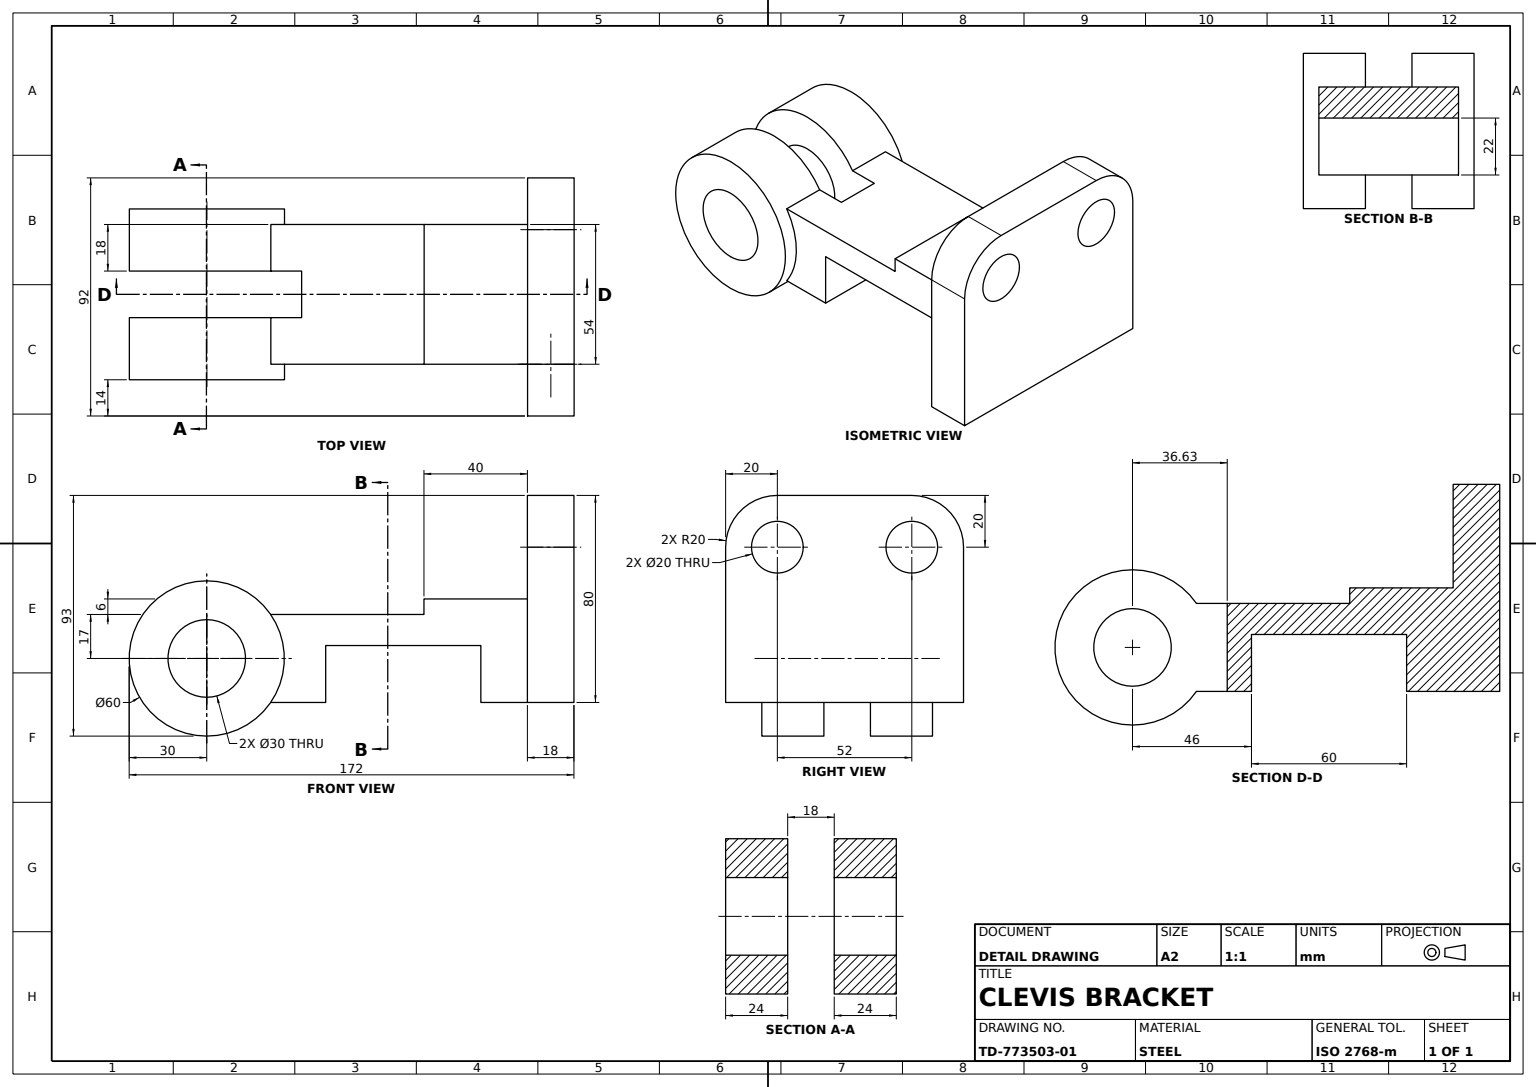
from build123d import *

# Parameters (mm, degrees)
MOUNTING_PLATE_SKETCH_R       = 10
MOUNTING_PLATE_DEPTH          = 18
ARM_START                     = -20
ARM_SKETCH_40X40_W            = 40
ARM_SKETCH_40X40_H            = 40
ARM_BOSS_DEPTH                = 54
ARM_EXTENSION_SKETCH_W        = 62
ARM_EXTENSION_SKETCH_H        = 34
ARM_EXTENSION_DEPTH           = 54
ARM_RECESS_SKETCH_W           = 60
ARM_RECESS_SKETCH_H           = 22
ARM_RECESS_CUT_DEPTH          = 54
STEP_PAD_DEPTH                = 6
STEP_PAD_DEPTH_BACK           = 60
STEP_PAD_SKETCH_R             = 30
STEP_PAD_SKETCH_R_2           = 15
CLEVIS_PROFILE_CUT_DEPTH      = 211.82694325
CLEVIS_PROFILE_CUT_DEPTH_BACK = 211.82694325
CLEVIS_PROFILE_SKETCH_W       = 18
CLEVIS_PROFILE_SKETCH_H       = 63.461103314
CLEVIS_SLOT_CUT_DEPTH         = 201.641471286
CLEVIS_SLOT_CUT_DEPTH_BACK    = 201.641471286
CLEVIS_SLOT_SKETCH_W          = 18
CLEVIS_SLOT_SKETCH_H          = 11.909045211


with BuildPart() as part:
    # Mounting Plate Sketch → Mounting Plate (new body)
    with BuildSketch(Plane.XY):
        with BuildLine():
            Line((0, 0), (92, 0))
            Line((92, 0), (92, 60))
            ThreePointArc((92, 60), (86.142135624, 74.142135624), (72, 80))
            Line((72, 80), (20, 80))
            ThreePointArc((20, 80), (5.857864376, 74.142135624), (0, 60))
            Line((0, 60), (0, 0))
        make_face()
        with Locations((20, 60)):
            Circle(MOUNTING_PLATE_SKETCH_R, mode=Mode.SUBTRACT)
        with Locations((72, 60)):
            Circle(MOUNTING_PLATE_SKETCH_R, mode=Mode.SUBTRACT)
    extrude(amount=MOUNTING_PLATE_DEPTH)

    # Arm Sketch 40x40 → Arm Boss (add)
    with BuildSketch(Plane(origin=(92, 0, 0), x_dir=(0, 0, -1), z_dir=(1, 0, 0)).offset(ARM_START)):
        with Locations((-38, 20)):
            Rectangle(ARM_SKETCH_40X40_W, ARM_SKETCH_40X40_H)
    extrude(amount=-ARM_BOSS_DEPTH)

    # Arm Extension Sketch → Arm Extension (add)
    with BuildSketch(Plane(origin=(72, 0, 0), x_dir=(0, 0, -1), z_dir=(1, 0, 0))):
        with Locations((-89, 17)):
            Rectangle(ARM_EXTENSION_SKETCH_W, ARM_EXTENSION_SKETCH_H)
    extrude(amount=-ARM_EXTENSION_DEPTH)

    # Arm Recess Sketch → Arm Recess Cut (cut)
    with BuildSketch(Plane(origin=(72, 0, 0), x_dir=(0, 0, -1), z_dir=(1, 0, 0))):
        with Locations((-66, 11)):
            Rectangle(ARM_RECESS_SKETCH_W, ARM_RECESS_SKETCH_H)
    extrude(amount=-ARM_RECESS_CUT_DEPTH, mode=Mode.SUBTRACT)

    # Step Pad Sketch → Step Pad (add, two sides: drawn at the far end of the back side and taken through both)
    with BuildSketch(Plane(origin=(72, 0, 0), x_dir=(0, 0, -1), z_dir=(1, 0, 0)).offset(-STEP_PAD_DEPTH_BACK)):
        with Locations(Location((-142, 17, 0), (0, 0, 90))):
            Circle(STEP_PAD_SKETCH_R)
        with Locations(Location((-142, 17, 0), (0, 0, 90))):
            Circle(STEP_PAD_SKETCH_R_2, mode=Mode.SUBTRACT)
    extrude(amount=STEP_PAD_DEPTH + STEP_PAD_DEPTH_BACK)

    # Clevis Profile Sketch → Clevis Profile Cut (cut, two sides: drawn at the far end of the back side and taken through both)
    with BuildSketch(Plane(origin=(0, 0, 0), x_dir=(1, 0, 0), z_dir=(0, 1, 0)).offset(-CLEVIS_PROFILE_CUT_DEPTH_BACK)):
        with Locations((45, -149.012137468)):
            Rectangle(CLEVIS_PROFILE_SKETCH_W, CLEVIS_PROFILE_SKETCH_H)
    extrude(amount=CLEVIS_PROFILE_CUT_DEPTH + CLEVIS_PROFILE_CUT_DEPTH_BACK, mode=Mode.SUBTRACT)

    # Clevis Slot Sketch → Clevis Slot Cut (cut, two sides: drawn at the far end of the back side and taken through both)
    with BuildSketch(Plane(origin=(0, 34, 0), x_dir=(1, 0, 0), z_dir=(0, 1, 0)).offset(-CLEVIS_SLOT_CUT_DEPTH_BACK)):
        with Locations((45, -111.327063206)):
            Rectangle(CLEVIS_SLOT_SKETCH_W, CLEVIS_SLOT_SKETCH_H)
    extrude(amount=CLEVIS_SLOT_CUT_DEPTH + CLEVIS_SLOT_CUT_DEPTH_BACK, mode=Mode.SUBTRACT)


solid = part.part
